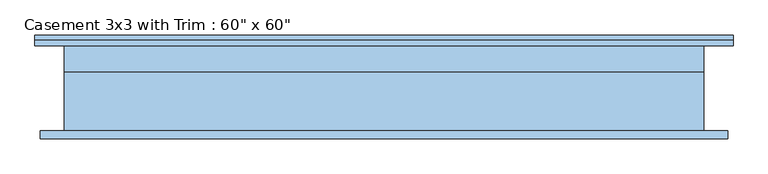
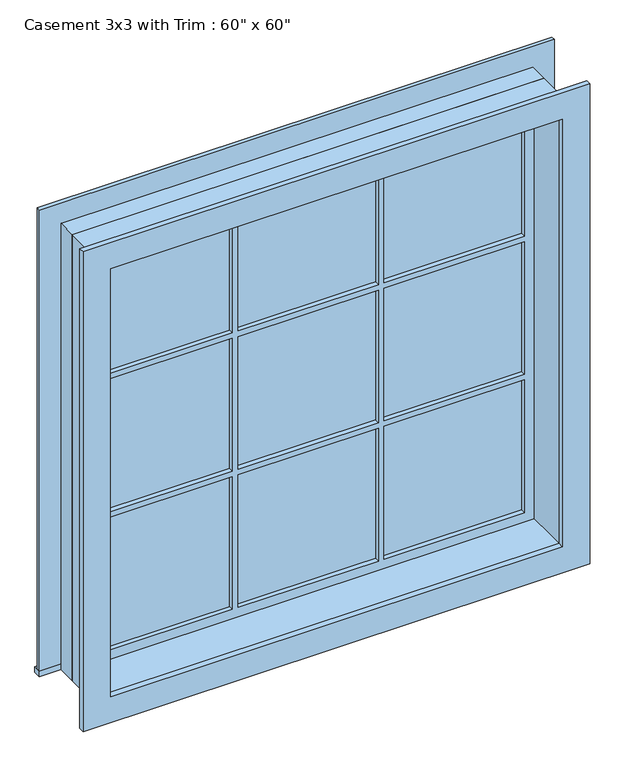
"""IFC4 building model written with IfcOpenShell, lengths in millimetres: window geometry."""

from ifc_helpers import new_model, si_unit, frame, origin, place, context, project, spatial, polyline, outline, extrude, source, transform, mapped, element, save


def window_8901c6e2(model_context):
    return source(origin(), model_context, "Body", "SweptSolid", [
        extrude(outline(polyline([(-831.85, 127.0), (831.85, 127.0), (831.85, 101.6), (-831.85, 101.6), (-831.85, 127.0)])), frame((0.0, 0.0, 304.8), z_axis=(0.0, 0.0, 1.0), x_axis=(1.0, 0.0, 0.0)), (0.0, 0.0, 1.0), 19.05),
        extrude(outline(polyline([(1809.75, -742.95), (1809.75, 742.95), (323.85, 742.95), (323.85, 831.85), (1898.65, 831.85), (1898.65, -831.85), (323.85, -831.85), (323.85, -742.95), (1809.75, -742.95)])), frame((0.0, 101.6, 0.0), z_axis=(0.0, 1.0, 0.0), x_axis=(0.0, 0.0, 1.0)), (0.0, 0.0, 1.0), 12.7),
        extrude(outline(polyline([(245.5333333, 66.675), (698.5, 66.675), (698.5, 53.975), (245.5333333, 53.975), (245.5333333, 66.675)])), frame((0.0, 0.0, 1312.3333333), z_axis=(0.0, 0.0, 1.0), x_axis=(1.0, 0.0, 0.0)), (0.0, 0.0, 1.0), 452.9666667),
        extrude(outline(polyline([(-226.4833333, 66.675), (226.4833333, 66.675), (226.4833333, 53.975), (-226.4833333, 53.975), (-226.4833333, 66.675)])), frame((0.0, 0.0, 1312.3333333), z_axis=(0.0, 0.0, 1.0), x_axis=(1.0, 0.0, 0.0)), (0.0, 0.0, 1.0), 452.9666667),
        extrude(outline(polyline([(-698.5, 66.675), (-245.5333333, 66.675), (-245.5333333, 53.975), (-698.5, 53.975), (-698.5, 66.675)])), frame((0.0, 0.0, 1312.3333333), z_axis=(0.0, 0.0, 1.0), x_axis=(1.0, 0.0, 0.0)), (0.0, 0.0, 1.0), 452.9666667),
        extrude(outline(polyline([(-698.5, 66.675), (-245.5333333, 66.675), (-245.5333333, 53.975), (-698.5, 53.975), (-698.5, 66.675)])), frame((0.0, 0.0, 840.3166667), z_axis=(0.0, 0.0, 1.0), x_axis=(1.0, 0.0, 0.0)), (0.0, 0.0, 1.0), 452.9666667),
        extrude(outline(polyline([(-226.4833333, 66.675), (226.4833333, 66.675), (226.4833333, 53.975), (-226.4833333, 53.975), (-226.4833333, 66.675)])), frame((0.0, 0.0, 840.3166667), z_axis=(0.0, 0.0, 1.0), x_axis=(1.0, 0.0, 0.0)), (0.0, 0.0, 1.0), 452.9666667),
        extrude(outline(polyline([(245.5333333, 66.675), (698.5, 66.675), (698.5, 53.975), (245.5333333, 53.975), (245.5333333, 66.675)])), frame((0.0, 0.0, 840.3166667), z_axis=(0.0, 0.0, 1.0), x_axis=(1.0, 0.0, 0.0)), (0.0, 0.0, 1.0), 452.9666667),
        extrude(outline(polyline([(245.5333333, 66.675), (698.5, 66.675), (698.5, 53.975), (245.5333333, 53.975), (245.5333333, 66.675)])), frame((0.0, 0.0, 368.3), z_axis=(0.0, 0.0, 1.0), x_axis=(1.0, 0.0, 0.0)), (0.0, 0.0, 1.0), 452.9666667),
        extrude(outline(polyline([(-226.4833333, 66.675), (226.4833333, 66.675), (226.4833333, 53.975), (-226.4833333, 53.975), (-226.4833333, 66.675)])), frame((0.0, 0.0, 368.3), z_axis=(0.0, 0.0, 1.0), x_axis=(1.0, 0.0, 0.0)), (0.0, 0.0, 1.0), 452.9666667),
        extrude(outline(polyline([(-698.5, 66.675), (-245.5333333, 66.675), (-245.5333333, 53.975), (-698.5, 53.975), (-698.5, 66.675)])), frame((0.0, 0.0, 368.3), z_axis=(0.0, 0.0, 1.0), x_axis=(1.0, 0.0, 0.0)), (0.0, 0.0, 1.0), 452.9666667),
        extrude(outline(polyline([(1885.95, 819.15), (1885.95, -819.15), (247.65, -819.15), (247.65, 819.15), (1885.95, 819.15)]), holes=[polyline([(1797.05, 730.25), (336.55, 730.25), (336.55, -730.25), (1797.05, -730.25), (1797.05, 730.25)])]), frame((0.0, -120.65, 0.0), z_axis=(0.0, 1.0, 0.0), x_axis=(0.0, 0.0, 1.0)), (0.0, 0.0, 1.0), 19.05),
        extrude(outline(polyline([(1809.75, -742.95), (323.85, -742.95), (323.85, 742.95), (1809.75, 742.95), (1809.75, -742.95)]), holes=[polyline([(1765.3, -245.5333333), (1312.3333333, -245.5333333), (1312.3333333, -698.5), (1765.3, -698.5), (1765.3, -245.5333333)]), polyline([(1293.2833333, -245.5333333), (840.3166667, -245.5333333), (840.3166667, -698.5), (1293.2833333, -698.5), (1293.2833333, -245.5333333)]), polyline([(821.2666667, -245.5333333), (368.3, -245.5333333), (368.3, -698.5), (821.2666667, -698.5), (821.2666667, -245.5333333)]), polyline([(1765.3, 226.4833333), (1312.3333333, 226.4833333), (1312.3333333, -226.4833333), (1765.3, -226.4833333), (1765.3, 226.4833333)]), polyline([(1293.2833333, 226.4833333), (840.3166667, 226.4833333), (840.3166667, -226.4833333), (1293.2833333, -226.4833333), (1293.2833333, 226.4833333)]), polyline([(821.2666667, 226.4833333), (368.3, 226.4833333), (368.3, -226.4833333), (821.2666667, -226.4833333), (821.2666667, 226.4833333)]), polyline([(1765.3, 698.5), (1312.3333333, 698.5), (1312.3333333, 245.5333333), (1765.3, 245.5333333), (1765.3, 698.5)]), polyline([(1293.2833333, 698.5), (840.3166667, 698.5), (840.3166667, 245.5333333), (1293.2833333, 245.5333333), (1293.2833333, 698.5)]), polyline([(821.2666667, 698.5), (368.3, 698.5), (368.3, 245.5333333), (821.2666667, 245.5333333), (821.2666667, 698.5)])]), frame((0.0, 38.1, 0.0), z_axis=(0.0, 1.0, 0.0), x_axis=(0.0, 0.0, 1.0)), (0.0, 0.0, 1.0), 44.45),
        extrude(outline(polyline([(1828.8, -762.0), (304.8, -762.0), (304.8, 762.0), (1828.8, 762.0), (1828.8, -762.0)]), holes=[polyline([(1797.05, -730.25), (1797.05, 730.25), (336.55, 730.25), (336.55, -730.25), (1797.05, -730.25)])]), frame((0.0, -101.6, 0.0), z_axis=(0.0, 1.0, 0.0), x_axis=(0.0, 0.0, 1.0)), (0.0, 0.0, 1.0), 139.7),
        extrude(outline(polyline([(1828.8, 762.0), (1828.8, -762.0), (304.8, -762.0), (304.8, 762.0), (1828.8, 762.0)]), holes=[polyline([(1809.75, 742.95), (323.85, 742.95), (323.85, -742.95), (1809.75, -742.95), (1809.75, 742.95)])]), frame((0.0, 38.1, 0.0), z_axis=(0.0, 1.0, 0.0), x_axis=(0.0, 0.0, 1.0)), (0.0, 0.0, 1.0), 63.5),
    ])


if __name__ == "__main__":
    model = new_model("IFC4")
    model_context = context("Model", 3, world=origin())
    ifc_project = project(units=[si_unit("LENGTHUNIT", "METRE", prefix="MILLI")], contexts=[model_context])
    site = spatial("IfcSite", under=ifc_project)
    building = spatial("IfcBuilding", under=site)
    placement = place(None, origin())
    window_shape = window_8901c6e2(model_context)
    element("IfcWindow", 1, ObjectType="Casement 3x3 with Trim : 60\" x 60\"", at=placement, inside=building, context=model_context, shape_type="MappedRepresentation", body=[
        mapped(window_shape, transform((0.0, 0.0, 0.0), x_axis=(1.0, 0.0, 0.0), y_axis=(0.0, 1.0, 0.0), z_axis=(0.0, 0.0, 1.0))),
    ])
    save(model, "model.ifc")

# Revit data of these elements
# Type "Casement 3x3 with Trim : 60\" x 60\""
#   Type Mark = "12"
#   Construction Type Id = "GSP4R"
#   Assembly Code = "B2020100"
#   Analytic Construction = "1/8 in Pilkington single glazing"
#   Visual Light Transmittance = 0.9
#   Solar Heat Gain Coefficient = 0.78
#   Heat Transfer Coefficient (U) = 0.6496 BTU/(h·ft²·°F)
#   Height = 5' - 0"
#   Default Sill Height = 1' - 0"
#   Trim Projection - Ext. = 0' - 0 1/2"
#   Trim Projection - Int. = 0' - 0 3/4"
#   Trim Width - Exterior = 0' - 3 1/2"
#   Trim Width - Interior = 0' - 3 1/2"
#   Width = 5' - 0"
#   Window Inset = 0' - 0 3/4"
#   Define Thermal Properties by = 1
#   Glass Pane Material = Glass
#   Sash Material = Sash
#   Trim Exterior Material = Trim
#   Trim Interior Material = Trim
#   Wall Closure = (empty or 0)
# Element 1 (IfcWindow, "Casement 3x3 with Trim : 60\" x 60\"")
#   Materials on its faces: "Sash", "Glass", "Trim"
# Materials
#   "Glass": class "Glass", colour RGB 0 128 192, transparency 0.75, Description = "Soda Lime Glass", Cost = 0
#   "Sash": class "Wood", colour RGB 224 178 126, transparency 0
#   "Trim": class "Wood", colour RGB 224 178 126, transparency 0
